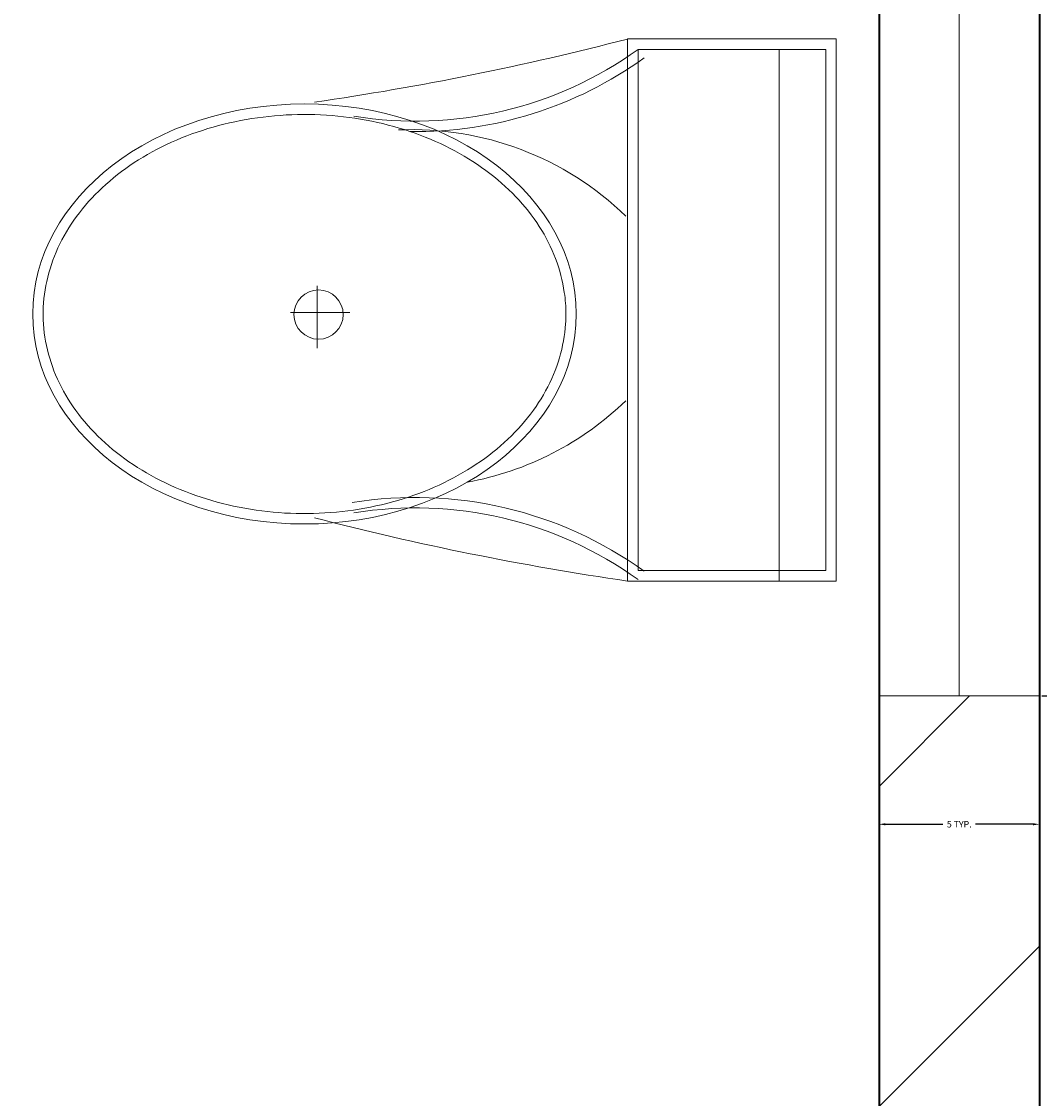
# Model space of a CAD drawing. Units: inches. Extents: x 1962 to 2771, y 1245 to 2660.
# Tile 82 of 114: x 2632 to 2661, y 2131 to 2161. Entities that reach past the tile are written whole.
import ezdxf

# ---------------------------------------------------------------- set-up
doc = ezdxf.new("R2010")
doc.units = ezdxf.units.IN
for name, color, linetype, lineweight in [('A-ANNO-DIMS', 2, 'Continuous', 18), ('A-FLOR-FIXT', 8, 'Continuous', 18), ('A-GLAZ', 4, 'Continuous', 18), ('A-WALL', 7, 'Continuous', 35), ('A-WALL-PATT', 252, 'Continuous', 13)]:
    doc.layers.add(name, color=color, linetype=linetype, lineweight=lineweight)
doc.styles.get("Standard").update_dxf_attribs({"font": 'arial.ttf'})
doc.dimstyles.get("Standard").update_dxf_attribs({"dimtxt": 0.18, "dimasz": 0.18, "dimexe": 0.18, "dimexo": 0.0625, "dimgap": 0.09, "dimtad": 0, "dimtih": 1, "dimtoh": 1, "dimdec": 4, "dimzin": 0, "dimdsep": 46, "dimtxsty": 'Standard', "dimcen": 0.09, "dimadec": 0, "dimazin": 0, "dimtfac": 1, "dimtdec": 4, "dimtofl": 0, "dimtmove": 0, "dimatfit": 3, "dimfxl": 1, "dimtolj": 1, "dimtzin": 0, "dimarcsym": 0})

# ---------------------------------------------------------------- blocks, each defined once
blk = doc.blocks.new('A$C31115884')
for p, q in [((257.5, 466.4), (257.5, 523.2)), ((283.1, 497.7), (223.4, 497.7)), ((0, 200), (0, 0)), ((520, 200), (0, 200)), ((520, 0), (520, 200)), ((10, 190), (10, 10)), ((510, 190), (10, 190)), ((510, 10), (510, 190)), ((510, 54.5), (0, 54.5)), ((10, 10), (510, 10)), ((0, 0), (520, 0))]:
    blk.add_line(p, q)
blk.add_circle((255.6, 496.4), 23.6)
for centre, radius, start, end in [((2777.7, -204.6), 2807, 165.4549, 171.7133), ((3237, 905), 2807, 188.2867, 194.5451), ((-294.5, 403.3), 364.7, 324.2091, 9.3499), ((-294.5, 403.3), 374.7, 324.2091, 9.3499), ((805.8, 403.3), 364.7, 170.6501, 215.7909), ((139.5, 406.2), 293.5, 315.8436, 2.6563), ((805.8, 403.3), 374.7, 179.2036, 215.7909), ((383.6, 406.2), 293.5, 190.2774, 224.1564)]:
    blk.add_arc(centre, radius, start, end)
blk.add_ellipse((256.2, 509.9), major_axis=(0, -260.7), ratio=0.772727)
blk.add_open_spline([(256.2, 259.2), (263.1, 259.2), (270, 259.7), (287.8, 262.3), (298.7, 265.1), (319.9, 273.1), (330.2, 278.4), (350.1, 291.1), (359.7, 298.7), (377.7, 315.9), (386.2, 325.5), (401.7, 346.6), (408.8, 358.1), (421.3, 382.5), (426.8, 395.5), (435.9, 422.4), (439.5, 436.4), (444.8, 465.1), (446.5, 479.7), (447.9, 509.2), (447.6, 524), (445, 553.3), (442.7, 567.8), (436.3, 596), (432.1, 609.7), (421.9, 636), (416, 648.6), (402.5, 672.1), (395, 683), (378.6, 703), (369.8, 712.1), (351.1, 728), (341.3, 734.8), (320.9, 746.2), (310.4, 750.7), (288.9, 757.3), (278, 759.4), (256, 761), (245, 760.6), (223.1, 757.2), (212.3, 754.3), (191.1, 746.1), (180.8, 740.7), (160.9, 727.8), (151.4, 720.1), (133.5, 702.7), (125.1, 693), (109.6, 671.7), (102.6, 660.2), (90.2, 635.7), (84.9, 622.7), (76, 595.6), (72.4, 581.6), (67.2, 552.9), (65.6, 538.2), (64.4, 508.8), (64.8, 494), (67.5, 464.7), (69.9, 450.2), (76.6, 422), (80.8, 408.3), (91.1, 382.2), (97.2, 369.7), (110.8, 346.3), (118.4, 335.4), (134.8, 315.6), (143.7, 306.7), (162.4, 290.9), (172.3, 284.2), (192.8, 273), (203.3, 268.6), (224.8, 262.2), (235.8, 260.2), (249.9, 259.3), (253, 259.2), (256.2, 259.2)], degree=3, knots=[0, 0, 0, 0, 0.110105, 0.110105, 0.285049, 0.285049, 0.459994, 0.459994, 0.634938, 0.634938, 0.809882, 0.809882, 0.984827, 0.984827, 1.159771, 1.159771, 1.334715, 1.334715, 1.50966, 1.50966, 1.684604, 1.684604, 1.859549, 1.859549, 2.034493, 2.034493, 2.209437, 2.209437, 2.384382, 2.384382, 2.559326, 2.559326, 2.73427, 2.73427, 2.909215, 2.909215, 3.084159, 3.084159, 3.259103, 3.259103, 3.434048, 3.434048, 3.608992, 3.608992, 3.783936, 3.783936, 3.958881, 3.958881, 4.133825, 4.133825, 4.30877, 4.30877, 4.483714, 4.483714, 4.658658, 4.658658, 4.833603, 4.833603, 5.008547, 5.008547, 5.183491, 5.183491, 5.358436, 5.358436, 5.53338, 5.53338, 5.708324, 5.708324, 5.883269, 5.883269, 6.058213, 6.058213, 6.233158, 6.233158, 6.283185, 6.283185, 6.283185, 6.283185])
blk = doc.blocks.new('WIN-24IN-B')
for p, q in [((0, 24), (4.5, 24)), ((4.5, 24), (2.25, 24)), ((2.25, 24), (2.25, 0)), ((4.5, 0), (0, 0)), ((2.25, 0), (4.5, 0))]:
    blk.add_line(p, q)
blk = doc.blocks.new('*D20')
at = {"layer": 'A-ANNO-DIMS', "color": 0, "lineweight": -2, "transparency": 16777216}
for p, q in [((2660.87, 2166.485), (2664.587, 2166.485)), ((2664.407, 2166.305), (2664.407, 2154.665)), ((2664.407, 2142.665), (2664.407, 2154.304)), ((2660.87, 2142.485), (2664.587, 2142.485))]:
    blk.add_line(p, q, dxfattribs=at)
at = {"layer": 'A-ANNO-DIMS', "color": 0, "transparency": 16777216}
for points in [[(2664.377, 2166.305), (2664.437, 2166.305), (2664.407, 2166.485)], [(2664.377, 2142.665), (2664.437, 2142.665), (2664.407, 2142.485)]]:
    blk.add_solid(points, dxfattribs=at)
at = {"layer": 'Defpoints', "color": 0, "transparency": 16777216}
for p in [(2660.807, 2166.485), (2664.407, 2166.485), (2660.807, 2142.485)]:
    blk.add_point(p, dxfattribs=at)
at = {"layer": 'A-ANNO-DIMS', "color": 0, "transparency": 16777216, "insert": (2664.407, 2154.485), "char_height": 0.18, "attachment_point": 5}
blk.add_mtext('\\A1;W1B 24 TYP.', dxfattribs=at)
blk = doc.blocks.new('*D21')
at = {"layer": 'A-ANNO-DIMS', "color": 0, "lineweight": -2, "transparency": 16777216}
for p, q in [((2656.307, 2142.422), (2656.307, 2138.705)), ((2660.807, 2142.422), (2660.807, 2138.705)), ((2656.487, 2138.885), (2658.099, 2138.885)), ((2660.627, 2138.885), (2659.016, 2138.885))]:
    blk.add_line(p, q, dxfattribs=at)
at = {"layer": 'A-ANNO-DIMS', "color": 0, "transparency": 16777216}
for points in [[(2656.487, 2138.915), (2656.487, 2138.855), (2656.307, 2138.885)], [(2660.627, 2138.915), (2660.627, 2138.855), (2660.807, 2138.885)]]:
    blk.add_solid(points, dxfattribs=at)
at = {"layer": 'Defpoints', "color": 0, "transparency": 16777216}
for p in [(2656.307, 2142.485), (2660.807, 2142.485), (2660.807, 2138.885)]:
    blk.add_point(p, dxfattribs=at)
at = {"layer": 'A-ANNO-DIMS', "color": 0, "transparency": 16777216, "insert": (2658.557, 2138.885), "char_height": 0.18, "attachment_point": 5}
blk.add_mtext('\\A1;5 TYP.', dxfattribs=at)
blk = doc.blocks.new('*D40')
at = {"layer": 'A-ANNO-DIMS', "color": 0, "lineweight": -2, "transparency": 16777216}
for p, q in [((2072.02, 2033.906), (2072.02, 2583.474)), ((2660.807, 2524.406), (2660.807, 2583.474)), ((2072.2, 2583.294), (2366.02, 2583.294)), ((2660.627, 2583.294), (2366.808, 2583.294))]:
    blk.add_line(p, q, dxfattribs=at)
at = {"layer": 'A-ANNO-DIMS', "color": 0, "transparency": 16777216}
for points in [[(2072.2, 2583.324), (2072.2, 2583.264), (2072.02, 2583.294)], [(2660.627, 2583.324), (2660.627, 2583.264), (2660.807, 2583.294)]]:
    blk.add_solid(points, dxfattribs=at)
at = {"layer": 'Defpoints', "color": 0, "transparency": 16777216}
for p in [(2660.807, 2583.294), (2660.807, 2524.344), (2072.02, 2033.844)]:
    blk.add_point(p, dxfattribs=at)
at = {"layer": 'A-ANNO-DIMS', "color": 0, "transparency": 16777216, "insert": (2366.414, 2583.294), "char_height": 0.18, "attachment_point": 5}
blk.add_mtext('\\A1;588.8', dxfattribs=at)

msp = doc.modelspace()

# ---------------------------------------------------------------- hatches: boundary and pattern name
at = {"layer": 'A-WALL-PATT'}
h = msp.add_hatch(dxfattribs=at)
h.set_pattern_fill('ANSI32', color=256)
h.paths.add_polyline_path([(2090.8074, 2467.3437), (2141.6481, 2467.3437), (2141.6481, 2469.5937), (2141.6481, 2471.8437), (2086.3074, 2471.8437), (2086.3074, 2422.5333), (2090.8074, 2422.5333)])
h.paths.add_polyline_path([(2282.7664, 2471.8437), (2204.8982, 2471.8437), (2204.8982, 2467.3437), (2234.8074, 2467.3437), (2234.8074, 2311.3437), (2228.7492, 2311.3437), (2228.7492, 2306.8437), (2234.8074, 2306.8437), (2331.9227, 2306.8437), (2331.9227, 2309.0937), (2331.9227, 2311.3437), (2239.3074, 2311.3437), (2239.3074, 2467.3437), (2282.7664, 2467.3437), (2282.7664, 2469.5937)])
h.paths.add_polyline_path([(2471.4531, 2519.8437), (2552.011, 2519.8437), (2564.3996, 2519.8437), (2564.3996, 2511.1389), (2568.8996, 2511.1389), (2568.8996, 2524.3437), (2466.9531, 2524.3437), (2466.9531, 2471.8437), (2450.0749, 2471.8437), (2446.4672, 2471.8437), (2446.4672, 2467.3437), (2450.0749, 2467.3437), (2475.9988, 2467.3437), (2475.9988, 2469.5937), (2475.9988, 2471.8437), (2471.4531, 2471.8437)])
h.paths.add_polyline_path([(2575.2231, 2469.5937), (2575.2231, 2471.8437), (2568.8996, 2471.8437), (2568.8996, 2487.1389), (2564.3996, 2487.1389), (2564.3996, 2471.8437), (2556.511, 2471.8437), (2499.2904, 2471.8437), (2499.2904, 2467.3437), (2507.8074, 2467.3437), (2507.8074, 2311.3437), (2414.863, 2311.3437), (2414.863, 2306.8437), (2512.3074, 2306.8437), (2517.0114, 2306.8437), (2517.0114, 2309.0937), (2517.0114, 2311.3437), (2512.3074, 2311.3437), (2512.3074, 2467.3437), (2575.2231, 2467.3437)])
h.paths.add_polyline_path([(2660.8074, 2471.8437), (2600.9602, 2471.8437), (2600.9602, 2467.3437), (2656.3074, 2467.3437), (2656.3074, 2432.5704), (2660.8074, 2432.5704)])
h.paths.add_polyline_path([(2660.8074, 2372.5704), (2656.3074, 2372.5704), (2656.3074, 2311.3437), (2600.276, 2311.3437), (2600.276, 2309.0937), (2600.276, 2306.8437), (2656.3074, 2306.8437), (2656.3074, 2296.2593), (2660.8074, 2296.2593)])
h.paths.add_polyline_path([(2572.3074, 2306.8437), (2577.1385, 2306.8437), (2577.1385, 2311.3437), (2551.082, 2311.3437), (2551.082, 2306.8437), (2567.8074, 2306.8437), (2567.8074, 2258.8437), (2540.0574, 2258.8437), (2540.0574, 2256.5937), (2540.0574, 2254.3437), (2567.8074, 2254.3437), (2656.3074, 2254.3437), (2656.3074, 2236.9085), (2660.8074, 2236.9085), (2660.8074, 2272.2593), (2656.3074, 2272.2593), (2656.3074, 2258.8437), (2572.3074, 2258.8437)])
h.paths.add_polyline_path([(2512.3074, 2254.3437), (2518.8716, 2254.3437), (2518.8716, 2256.5937), (2518.8716, 2258.8437), (2507.8074, 2258.8437), (2507.8074, 2177.8437), (2567.8074, 2177.8437), (2567.8074, 2172.9628), (2572.3074, 2172.9628), (2572.3074, 2177.8437), (2656.3074, 2177.8437), (2656.3074, 2166.4846), (2660.8074, 2166.4846), (2660.8074, 2200.9085), (2656.3074, 2200.9085), (2656.3074, 2182.3437), (2512.3074, 2182.3437)])
h.paths.add_polyline_path([(2656.3074, 2129.8437), (2572.3074, 2129.8437), (2572.3074, 2150.3044), (2570.0574, 2150.3044), (2567.8074, 2150.3044), (2567.8074, 2129.8437), (2507.8074, 2129.8437), (2507.8074, 2116.3027), (2510.0574, 2116.3027), (2512.3074, 2116.3027), (2512.3074, 2125.3437), (2567.8074, 2125.3437), (2572.3074, 2125.3437), (2656.3074, 2125.3437)])
h.paths.add_polyline_path([(2090.8074, 2362.5333), (2086.3074, 2362.5333), (2086.3074, 2298.6242), (2090.8074, 2298.6242), (2090.8074, 2306.8437), (2174.8074, 2306.8437), (2174.8074, 2286.4178), (2179.3074, 2286.4178), (2179.3074, 2306.8437), (2192.8641, 2306.8437), (2192.8641, 2309.0937), (2192.8641, 2311.3437), (2090.8074, 2311.3437)])
h.paths.add_polyline_path([(2209.156, 2258.8437), (2179.3074, 2258.8437), (2179.3074, 2263.2236), (2177.0574, 2263.2236), (2174.8074, 2263.2236), (2174.8074, 2258.8437), (2090.8074, 2258.8437), (2090.8074, 2274.6242), (2086.3074, 2274.6242), (2086.3074, 2238.2967), (2088.5574, 2238.2967), (2090.8074, 2238.2967), (2090.8074, 2254.3437), (2209.156, 2254.3437)])
h.paths.add_polyline_path([(2090.8074, 2177.8437), (2234.8074, 2177.8437), (2234.8074, 2173.1428), (2239.3074, 2173.1428), (2239.3074, 2258.8437), (2230.8442, 2258.8437), (2230.8442, 2256.5937), (2230.8442, 2254.3437), (2234.8074, 2254.3437), (2234.8074, 2182.3437), (2090.8074, 2182.3437), (2090.8074, 2202.2967), (2086.3074, 2202.2967), (2086.3074, 2140.0389), (2090.8074, 2140.0389)])
h.paths.add_polyline_path([(2090.8074, 2080.0389), (2086.3074, 2080.0389), (2086.3074, 2033.8437), (2090.8074, 2033.8437)], flags=17)
h.paths.add_polyline_path([(2244.9405, 2033.8437), (2239.3074, 2033.8437), (2239.3074, 2142.0665), (2237.2592, 2142.0665), (2234.8074, 2142.0665), (2234.8074, 2033.8437), (2090.8074, 2033.8437), (2076.5204, 2033.8437), (2072.0204, 2033.8437), (2072.0204, 2000.4493), (2076.5204, 2000.4493), (2076.5204, 2029.3437), (2090.8074, 2029.3437), (2244.9405, 2029.3437), (2244.9405, 2031.5937)])
h.paths.add_polyline_path([(2234.8074, 1933.3437), (2076.5204, 1933.3437), (2076.5204, 1952.4493), (2074.2704, 1952.4493), (2072.0204, 1952.4493), (2072.0204, 1933.3437), (2072.0204, 1928.8437), (2234.8074, 1928.8437)])
h.paths.add_polyline_path([(2090.8074, 1928.8437), (2086.3074, 1928.8437), (2086.3074, 1906.5013), (2090.8074, 1906.5013)])
h.paths.add_polyline_path([(2090.8074, 1846.5013), (2086.3074, 1846.5013), (2086.3074, 1769.9917), (2088.5574, 1769.9917), (2090.8074, 1769.9917), (2090.8074, 1780.3437), (2234.8074, 1780.3437), (2234.8074, 1708.3437), (2230.3764, 1708.3437), (2230.3764, 1703.8437), (2239.3074, 1703.8437), (2239.3074, 1792.6669), (2237.0574, 1792.6669), (2234.8074, 1792.6669), (2234.8074, 1784.8437), (2090.8074, 1784.8437)])
h.paths.add_polyline_path([(2239.3074, 1928.8437), (2244.9405, 1928.8437), (2244.9405, 1931.0937), (2244.9405, 1933.3437), (2234.8074, 1933.3437), (2234.8074, 1928.8437), (2234.8074, 1825.5949), (2239.3074, 1825.5949)])
h.paths.add_polyline_path([(2148.0425, 1649.0937), (2148.0425, 1651.3437), (2090.8074, 1651.3437), (2090.8074, 1646.8437), (2148.0425, 1646.8437)], flags=0)
h.paths.add_polyline_path([(2207.5601, 1708.3437), (2090.8074, 1708.3437), (2090.8074, 1703.8437), (2174.8074, 1703.8437), (2174.8074, 1651.3437), (2170.4457, 1651.3437), (2170.4457, 1646.8437), (2195.9924, 1646.8437), (2195.9924, 1649.0937), (2195.9924, 1651.3437), (2179.3074, 1651.3437), (2179.3074, 1703.8437), (2207.5601, 1703.8437), (2207.5601, 1706.0937)])
h.paths.add_polyline_path([(2090.8074, 1733.9917), (2086.3074, 1733.9917), (2086.3074, 1696.1032), (2088.5574, 1696.1032), (2090.8074, 1696.1032)])
h.paths.add_polyline_path([(2090.8074, 1672.1032), (2086.3074, 1672.1032), (2086.3074, 1600.3335), (2090.8074, 1600.3335)])
h.paths.add_polyline_path([(2090.8074, 1540.3335), (2086.3074, 1540.3335), (2086.3074, 1486.3437), (2139.6766, 1486.3437), (2139.6766, 1490.8437), (2090.8074, 1490.8437)])
h.paths.add_polyline_path([(2302.3876, 1490.8437), (2239.3074, 1490.8437), (2239.3074, 1646.8437), (2335.9994, 1646.8437), (2335.9994, 1651.3437), (2229.884, 1651.3437), (2229.884, 1646.8437), (2234.8074, 1646.8437), (2234.8074, 1490.8437), (2202.7103, 1490.8437), (2202.7103, 1488.5937), (2202.7103, 1486.3437), (2275.0699, 1486.3437), (2275.0699, 1475.772), (2279.5699, 1475.772), (2279.5699, 1486.3437), (2302.3876, 1486.3437)])
h.paths.add_polyline_path([(2279.5699, 1451.772), (2275.0699, 1451.772), (2275.0699, 1438.3437), (2174.8074, 1438.3437), (2174.8074, 1486.3437), (2179.7922, 1486.3437), (2179.7922, 1490.8437), (2163.3585, 1490.8437), (2163.3585, 1488.5937), (2163.3585, 1486.3437), (2170.3074, 1486.3437), (2170.3074, 1433.8437), (2279.5699, 1433.8437)])
h.paths.add_polyline_path([(2427.2363, 1490.8437), (2375.8074, 1490.8437), (2375.8074, 1646.8437), (2381.6401, 1646.8437), (2381.6401, 1651.3437), (2365.887, 1651.3437), (2365.887, 1649.0937), (2365.887, 1646.8437), (2371.3074, 1646.8437), (2371.3074, 1490.8437), (2327.5627, 1490.8437), (2327.5627, 1488.5937), (2327.5627, 1486.3437), (2371.3074, 1486.3437), (2371.3074, 1433.8437), (2375.8074, 1433.8437), (2375.8074, 1486.3437), (2427.2363, 1486.3437)])
h.paths.add_polyline_path([(2512.3074, 1646.8437), (2519.4351, 1646.8437), (2519.4351, 1649.0937), (2519.4351, 1651.3437), (2507.8074, 1651.3437), (2416.0063, 1651.3437), (2416.0063, 1649.0937), (2416.0063, 1646.8437), (2507.8074, 1646.8437), (2507.8074, 1490.8437), (2497.0532, 1490.8437), (2497.0532, 1488.5937), (2497.0532, 1486.3437), (2574.9344, 1486.3437), (2574.9344, 1476.0181), (2579.4344, 1476.0181), (2579.4344, 1486.3437), (2584.4872, 1486.3437), (2584.3074, 1490.8437), (2512.3074, 1490.8437)])
h.paths.add_polyline_path([(2470.5091, 1486.3437), (2473.9767, 1486.3437), (2473.9767, 1490.8437), (2449.6605, 1490.8437), (2449.6605, 1488.5937), (2449.6605, 1486.3437), (2466.0091, 1486.3437), (2466.0091, 1433.8437), (2470.5091, 1433.8437), (2579.4344, 1433.8437), (2579.4344, 1452.0181), (2574.9344, 1452.0181), (2574.9344, 1438.3437), (2554.5091, 1438.3437), (2470.5091, 1438.3437)])
h.paths.add_polyline_path([(2656.3074, 1490.8437), (2611.86, 1490.8437), (2611.86, 1486.3437), (2656.3074, 1486.3437)])
h.paths.add_polyline_path([(2660.8074, 1532.7007), (2658.5574, 1532.7007), (2656.3074, 1532.7007), (2656.3074, 1486.3437), (2660.8074, 1486.3437)])
h.paths.add_polyline_path([(2660.8074, 1664.9663), (2656.3074, 1664.9663), (2656.3074, 1651.3437), (2602.2313, 1651.3437), (2602.2313, 1646.8437), (2656.3074, 1646.8437), (2656.3074, 1592.7007), (2660.8074, 1592.7007)])
h.paths.add_polyline_path([(2660.8074, 1724.5221), (2656.3074, 1724.5221), (2656.3074, 1703.8437), (2542.4725, 1703.8437), (2542.4725, 1699.3437), (2567.8074, 1699.3437), (2567.8074, 1651.3437), (2552.7766, 1651.3437), (2552.7766, 1649.0937), (2552.7766, 1646.8437), (2577.2878, 1646.8437), (2577.2878, 1649.0937), (2577.2878, 1651.3437), (2572.3074, 1651.3437), (2572.3074, 1699.3437), (2656.3074, 1699.3437), (2656.3074, 1688.9663), (2660.8074, 1688.9663)])
h.paths.add_polyline_path([(2660.8074, 1880.6524), (2656.3074, 1880.6524), (2656.3074, 1832.8437), (2512.3074, 1832.8437), (2512.3074, 1837.8959), (2507.8074, 1837.8959), (2507.8074, 1828.3437), (2567.8074, 1828.3437), (2567.8074, 1804.3437), (2572.3074, 1804.3437), (2572.3074, 1828.3437), (2656.3074, 1828.3437), (2656.3074, 1818.6778), (2660.8074, 1818.6778)])
h.paths.add_polyline_path([(2660.8074, 1794.6778), (2656.3074, 1794.6778), (2656.3074, 1780.3437), (2572.3074, 1780.3437), (2572.3074, 1783.0303), (2570.0574, 1783.0303), (2567.8074, 1783.0303), (2567.8074, 1780.3437), (2507.8074, 1780.3437), (2507.8074, 1699.3437), (2517.8858, 1699.3437), (2517.8858, 1701.5937), (2517.8858, 1703.8437), (2512.3074, 1703.8437), (2512.3074, 1775.8437), (2656.3074, 1775.8437), (2656.3074, 1760.5221), (2660.8074, 1760.5221)])
h.paths.add_polyline_path([(2660.8074, 1981.3437), (2660.8074, 2020.2808), (2658.5574, 2020.2808), (2656.3074, 2020.2808), (2656.3074, 1981.3437), (2512.3074, 1981.3437), (2512.3074, 2086.6996), (2507.8074, 2086.6996), (2507.8074, 1981.3437), (2375.8074, 1981.3437), (2375.8074, 1986.8505), (2373.5574, 1986.8505), (2371.3074, 1986.8505), (2371.3074, 1973.2607), (2375.8074, 1973.2607), (2375.8074, 1976.8437), (2507.8074, 1976.8437), (2507.8074, 1865.4281), (2510.0574, 1865.4281), (2512.3074, 1865.4281), (2512.3074, 1976.8437), (2660.8074, 1976.8437)])
h.paths.add_polyline_path([(2375.8074, 1940.297), (2373.5574, 1940.297), (2371.3074, 1940.297), (2371.3074, 1933.3437), (2278.4434, 1933.3437), (2278.4434, 1928.8437), (2371.3074, 1928.8437), (2371.3074, 1651.3437), (2375.8074, 1651.3437)])
h.paths.add_polyline_path([(2660.8074, 1976.8437), (2656.3074, 1976.8437), (2656.3074, 1940.6524), (2660.8074, 1940.6524)], flags=17)
h.paths.add_polyline_path([(2660.8074, 2142.4846), (2656.3074, 2142.4846), (2656.3074, 2080.2808), (2660.8074, 2080.2808)])
h.paths.add_polyline_path([(2381.4189, 2311.3437), (2375.8074, 2311.3437), (2375.8074, 2467.3437), (2424.7242, 2467.3437), (2424.7242, 2469.5937), (2424.7242, 2471.8437), (2375.8074, 2471.8437), (2375.8074, 2524.3437), (2371.3074, 2524.3437), (2371.3074, 2471.8437), (2307.2097, 2471.8437), (2307.2097, 2467.3437), (2371.3074, 2467.3437), (2371.3074, 2311.3437), (2366.8901, 2311.3437), (2366.8901, 2306.8437), (2371.3074, 2306.8437), (2371.3074, 2033.8437), (2279.6589, 2033.8437), (2279.6589, 2029.3437), (2371.3074, 2029.3437), (2371.3074, 2014.2598), (2375.8074, 2014.2598), (2375.8074, 2306.8437), (2381.4189, 2306.8437)])
h.paths.add_polyline_path([(2263.3074, 2524.3437), (2170.3074, 2524.3437), (2170.3074, 2519.8437), (2170.3074, 2471.8437), (2165.0312, 2471.8437), (2165.0312, 2467.3437), (2179.6721, 2467.3437), (2179.6721, 2469.5161), (2179.6721, 2471.8437), (2174.8074, 2471.8437), (2174.8074, 2519.8437), (2258.8074, 2519.8437), (2258.8074, 2511.6436), (2263.3074, 2511.6436)])
h.paths.add_polyline_path([(2245.0232, 1361.4123), (2492.9468, 1361.4123), (2492.9468, 1398.505), (2245.0232, 1398.505)], flags=9)
h.paths.add_polyline_path([(2388.1434, 2086.6936), (2425.0704, 2086.6936), (2425.0704, 2105.3509), (2388.1434, 2105.3509)], flags=9)
h.paths.add_polyline_path([(2404.922, 2242.6744), (2445.7337, 2242.6744), (2445.7337, 2261.3318), (2404.922, 2261.3318)], flags=9)
h.paths.add_polyline_path([(2269.4107, 2156.7935), (2306.3378, 2156.7935), (2306.3378, 2175.4508), (2269.4107, 2175.4508)], flags=9)
h.paths.add_polyline_path([(2269.3277, 2233.4343), (2306.2547, 2233.4343), (2306.2547, 2252.0917), (2269.3277, 2252.0917)], flags=9)
h.paths.add_polyline_path([(2431.6052, 2320.6922), (2470.4456, 2320.6922), (2470.4456, 2339.3495), (2431.6052, 2339.3495)], flags=25)
h.paths.add_polyline_path([(2249.6902, 2315.7608), (2288.5306, 2315.7608), (2288.5306, 2334.4182), (2249.6902, 2334.4182)], flags=25)
h.paths.add_polyline_path([(2096.9301, 2314.3181), (2135.7704, 2314.3181), (2135.7704, 2332.9755), (2096.9301, 2332.9755)], flags=25)
h.paths.add_polyline_path([(2134.3475, 2285.7089), (2161.4655, 2285.7089), (2161.4655, 2304.3662), (2134.3475, 2304.3662)], flags=9)
h.paths.add_polyline_path([(2126.5155, 2209.4076), (2159.9227, 2209.4076), (2159.9227, 2228.065), (2126.5155, 2228.065)], flags=25)
h.paths.add_polyline_path([(2110.5753, 2141.5299), (2149.4157, 2141.5299), (2149.4157, 2160.1872), (2110.5753, 2160.1872)], flags=25)
h.paths.add_polyline_path([(2249.8618, 1968.3317), (2286.3966, 1968.3317), (2286.3966, 1986.989), (2249.8618, 1986.989)], flags=9)
h.paths.add_polyline_path([(2395.9507, 1777.0051), (2436.7624, 1777.0051), (2436.7624, 1795.6625), (2395.9507, 1795.6625)], flags=9)
h.paths.add_polyline_path([(2398.5259, 1888.5651), (2435.0062, 1888.5651), (2435.0062, 1907.2224), (2398.5259, 1907.2224)], flags=25)
h.paths.add_polyline_path([(2259.3506, 1728.3559), (2296.2776, 1728.3559), (2296.2776, 1747.0132), (2259.3506, 1747.0132)], flags=9)
h.paths.add_polyline_path([(2271.3698, 1845.268), (2308.2968, 1845.268), (2308.2968, 1863.9253), (2271.3698, 1863.9253)], flags=9)
h.paths.add_polyline_path([(2120.9355, 1786.3027), (2159.7759, 1786.3027), (2159.7759, 1804.9601), (2120.9355, 1804.9601)], flags=25)
h.paths.add_polyline_path([(2121.3164, 1732.1043), (2154.7236, 1732.1043), (2154.7236, 1750.7616), (2121.3164, 1750.7616)], flags=25)
h.paths.add_polyline_path([(2118.3706, 1678.8997), (2147.5282, 1678.8997), (2147.5282, 1697.557), (2118.3706, 1697.557)], flags=25)
h.paths.add_polyline_path([(2385.9227, 1493.557), (2424.763, 1493.557), (2424.763, 1512.2143), (2385.9227, 1512.2143)], flags=25)
h.paths.add_polyline_path([(2248.7058, 1500.0256), (2287.5462, 1500.0256), (2287.5462, 1518.6829), (2248.7058, 1518.6829)], flags=25)
h.paths.add_polyline_path([(2104.1669, 1617.3771), (2143.0073, 1617.3771), (2143.0073, 1636.0344), (2104.1669, 1636.0344)], flags=9)
h.paths.add_polyline_path([(2096.0714, 1447.8824), (2137.3845, 1447.8824), (2137.3845, 1458.1859), (2096.0714, 1458.1859)], flags=9)
h.paths.add_polyline_path([(2180.6114, 1440.325), (2209.7689, 1440.325), (2209.7689, 1458.9823), (2180.6114, 1458.9823)], flags=25)
h.paths.add_polyline_path([(2316.1698, 1447.9637), (2357.4829, 1447.9637), (2357.4829, 1458.2673), (2316.1698, 1458.2673)], flags=9)
h.paths.add_polyline_path([(2397.6187, 1447.9637), (2438.9318, 1447.9637), (2438.9318, 1458.2673), (2397.6187, 1458.2673)], flags=9)
h.paths.add_polyline_path([(2473.0778, 1439.5953), (2502.2354, 1439.5953), (2502.2354, 1458.2527), (2473.0778, 1458.2527)], flags=25)
h.paths.add_polyline_path([(2589.7027, 1447.8819), (2631.0158, 1447.8819), (2631.0158, 1458.1855), (2589.7027, 1458.1855)], flags=9)
h.paths.add_polyline_path([(2522.4009, 1497.5285), (2561.2413, 1497.5285), (2561.2413, 1516.1859), (2522.4009, 1516.1859)], flags=25)
h.paths.add_polyline_path([(2579.6565, 1671.3482), (2608.8141, 1671.3482), (2608.8141, 1690.0056), (2579.6565, 1690.0056)], flags=25)
h.paths.add_polyline_path([(2544.7038, 1725.5064), (2578.1111, 1725.5064), (2578.1111, 1744.1637), (2544.7038, 1744.1637)], flags=25)
h.paths.add_polyline_path([(2578.1191, 1807.472), (2607.2766, 1807.472), (2607.2766, 1826.1293), (2578.1191, 1826.1293)], flags=25)
h.paths.add_polyline_path([(2595.0614, 1835.1839), (2633.9018, 1835.1839), (2633.9018, 1853.8413), (2595.0614, 1853.8413)], flags=25)
h.paths.add_polyline_path([(2567.0097, 2097.7035), (2605.8501, 2097.7035), (2605.8501, 2116.3609), (2567.0097, 2116.3609)], flags=9)
h.paths.add_polyline_path([(2586.644, 2134.6454), (2615.8015, 2134.6454), (2615.8015, 2153.3027), (2586.644, 2153.3027)], flags=9)
h.paths.add_polyline_path([(2544.6185, 2212.6783), (2578.0258, 2212.6783), (2578.0258, 2231.3356), (2544.6185, 2231.3356)], flags=25)
h.paths.add_polyline_path([(2577.0273, 2256.9023), (2606.1849, 2256.9023), (2606.1849, 2275.5597), (2577.0273, 2275.5597)], flags=24)
h.paths.add_polyline_path([(2605.2683, 2315.2821), (2644.1087, 2315.2821), (2644.1087, 2333.9395), (2605.2683, 2333.9395)], flags=25)
h.paths.add_polyline_path([(2583.1244, 2496.1815), (2624.4375, 2496.1815), (2624.4375, 2506.4851), (2583.1244, 2506.4851)], flags=9)
h.paths.add_polyline_path([(2474.761, 2497.0823), (2503.9185, 2497.0823), (2503.9185, 2515.7397), (2474.761, 2515.7397)], flags=25)
h.paths.add_polyline_path([(2387.5787, 2494.2563), (2428.902, 2494.2563), (2428.902, 2504.5598), (2387.5787, 2504.5598)], flags=9)
h.paths.add_polyline_path([(2300.1657, 2500.1564), (2341.4788, 2500.1564), (2341.4788, 2510.46), (2300.1657, 2510.46)], flags=25)
h.paths.add_polyline_path([(2176.8589, 2497.5843), (2206.0165, 2497.5843), (2206.0165, 2516.2416), (2176.8589, 2516.2416)], flags=25)
h.paths.add_polyline_path([(2097.4668, 2494.9762), (2138.7799, 2494.9762), (2138.7799, 2505.2798), (2097.4668, 2505.2798)], flags=9)

# ---------------------------------------------------------------- linework, layer by layer
at = {"layer": 'A-WALL'}
for p, q in [((2660.8074, 2471.8437), (2660.8074, 1976.8437)), ((2656.3074, 2177.8437), (2656.3074, 1981.3437))]:
    msp.add_line(p, q, dxfattribs=at)

# ---------------------------------------------------------------- block references
at = {"layer": 'A-FLOR-FIXT', "xscale": 0.0292470664339069, "yscale": 0.0292470664339069, "zscale": 0.0292470664339069, "rotation": 89.99999999999999}
msp.add_blockref('A$C31115884', (2655.1034, 2145.7089), dxfattribs=at)
at = {"layer": 'A-GLAZ'}
msp.add_blockref('WIN-24IN-B', (2656.3074, 2142.4846), dxfattribs=at)

# ---------------------------------------------------------------- dimensions: what is measured, and where the dimension line sits
at = {"layer": 'A-ANNO-DIMS'}
dim = msp.add_linear_dim(base=(2660.8074, 2583.2937), p1=(2072.0204, 2033.8437), p2=(2660.8074, 2524.3437), dimstyle='Standard', override={"dimdec": 1, "dimlfac": 1, "dimrnd": 0, "dimzin": 0, "dimdsep": 46, "dimlunit": 2}, dxfattribs=at)
dim.commit()
dim.dimension.update_dxf_attribs({"geometry": '*D40', "text_midpoint": (2366.4139, 2583.2937)})
dim = msp.add_linear_dim(base=(2664.4074, 2166.4846), p1=(2660.8074, 2142.4846), p2=(2660.8074, 2166.4846), angle=90, text='W1B <> TYP.', dimstyle='Standard', override={"dimdec": 0, "dimlfac": 1, "dimrnd": 0, "dimzin": 0, "dimdsep": 46, "dimlunit": 2}, dxfattribs=at)
dim.commit()
dim.dimension.update_dxf_attribs({"geometry": '*D20', "text_midpoint": (2664.4074, 2154.4846)})
dim = msp.add_linear_dim(base=(2660.8073805882, 2138.8845600367), p1=(2656.3073805882, 2142.4845600367), p2=(2660.8073805882, 2142.4845600367), text='<> TYP.', dimstyle='Standard', override={"dimdec": 0, "dimlfac": 1, "dimrnd": 0, "dimzin": 0, "dimdsep": 46, "dimlunit": 2}, dxfattribs=at)
dim.commit()
dim.dimension.update_dxf_attribs({"geometry": '*D21', "text_midpoint": (2658.5573805882, 2138.8845600367)})

doc.saveas('drawing.dxf')
